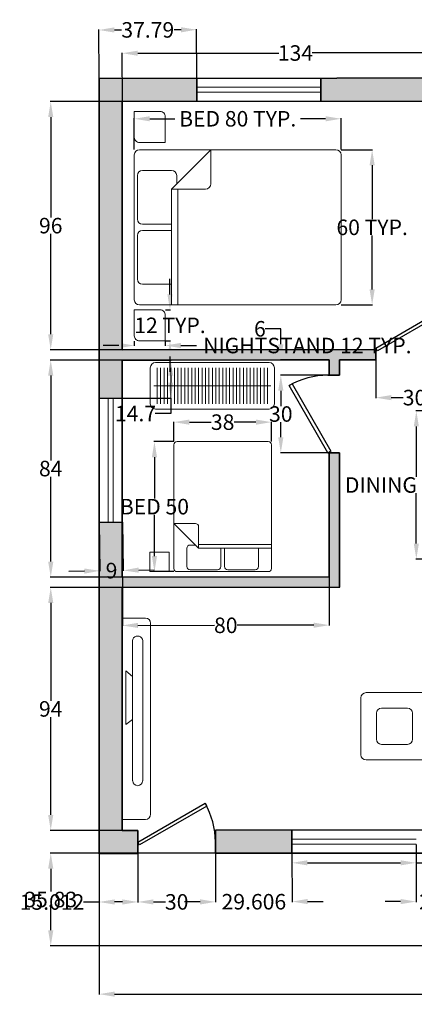
# Model space of a CAD drawing. Units: inches. Extents: x 98 to 487, y -240 to 141.
# Tile 1 of 5: x 98 to 251, y -240 to 141. Entities that reach past the tile are written whole.
import ezdxf

# ---------------------------------------------------------------- set-up
doc = ezdxf.new("R2010")
doc.units = ezdxf.units.IN
doc.header["$MEASUREMENT"] = 0
for name, color, linetype, lineweight in [('A-ANNO-DIMS', 2, 'Continuous', 18), ('A-DOOR', 3, 'Continuous', 25), ('A-EQPM', 9, 'Continuous', 18), ('A-FURN', 8, 'Continuous', 18), ('A-GLAZ', 4, 'Continuous', 18), ('A-WALL', 7, 'Continuous', 35)]:
    doc.layers.add(name, color=color, linetype=linetype, lineweight=lineweight)
doc.layers.add('A-WALL-PATT', color=251, linetype='Continuous', lineweight=13, true_color=0x636466)
doc.styles.get("Standard").update_dxf_attribs({"font": 'arial.ttf'})
doc.dimstyles.get("Standard").update_dxf_attribs({"dimtxt": 6, "dimasz": 6, "dimexe": 0.18, "dimexo": 0.0625, "dimgap": 0.09, "dimtad": 0, "dimtih": 1, "dimtoh": 1, "dimdec": 0, "dimzin": 0, "dimdsep": 46, "dimlunit": 4, "dimtxsty": 'Standard', "dimcen": 0.09, "dimadec": 0, "dimazin": 0, "dimtfac": 1, "dimtdec": 0, "dimtofl": 0, "dimtmove": 0, "dimatfit": 3, "dimfxl": 1, "dimtolj": 1, "dimtzin": 0, "dimarcsym": 0})

# ---------------------------------------------------------------- blocks, each defined once
blk = doc.blocks.new('Bed - Queen')
for p, q in [((2, 0), (57.99999, 0)), ((0, -78.00003), (0, -2)), ((7.99999, -14.4), (7.99999, -3.2)), ((9.99999, -1.2), (26.79998, -1.2)), ((28.79998, -3.2), (28.79998, -14.4)), ((31.19999, -14.4), (31.19999, -3.2)), ((33.19999, -1.2), (49.99999, -1.2)), ((51.99999, -3.2), (51.99999, -14.4)), ((59.99999, -2), (59.99999, -78.00003)), ((0, -14.4), (44.8, -14.4)), ((59.99999, -29.6), (44.8, -14.4)), ((44.8, -14.4), (44.8, -27.6)), ((44.8, -16.8), (0, -16.8)), ((49.99999, -16.4), (46.79936, -16.4)), ((46.8, -29.6), (59.99999, -29.6)), ((57.99999, -80.00003), (2, -80.00003))]:
    blk.add_line(p, q)
for centre, start, end in [((2, -2), 90, 180), ((57.99999, -2), 0, 90), ((9.99999, -3.2), 90, 180), ((26.79998, -3.2), 0, 90), ((33.19999, -3.2), 90, 180), ((49.99999, -3.2), 0, 90), ((49.99999, -14.4), 270, 0), ((46.8, -27.6), 180, 270), ((2, -78.00003), 180, 270), ((57.99999, -78.00003), 270, 0)]:
    blk.add_arc(centre, 2, start, end)
blk = doc.blocks.new('*U8')
for p, q in [((0, 0), (0, -6)), ((40, 0), (40, -6))]:
    blk.add_line(p, q)
blk.add_lwpolyline([(0, 0), (34.64, 20), (35.52, 18.48), (0.87, -1.52)], close=True)
blk.add_arc((0, 0), 40, 0, 30)
blk = doc.blocks.new('GLAZ-48IN')
for p, q in [((48, 2), (0, 2)), ((48, 0), (0, 0))]:
    blk.add_line(p, q)
blk = doc.blocks.new('NIGHTSTAND-12IN-RADIUSED')
blk.add_lwpolyline([(2, 0), (12, 0), (12, 10, 0.414214), (10, 12), (0, 12), (0, 2, 0.414214)], format="xyb", close=True)
blk = doc.blocks.new('WARDROBE-HANGING-RAIL')
for p, q in [((7, 46.67), (7, 1.33)), ((14, 45.33), (0, 45.33)), ((14, 44), (0, 44)), ((14, 42.67), (0, 42.67)), ((14, 41.33), (0, 41.33)), ((14, 40), (0, 40)), ((14, 38.67), (0, 38.67)), ((14, 37.33), (0, 37.33)), ((14, 36), (0, 36)), ((14, 34.67), (0, 34.67)), ((14, 33.33), (0, 33.33)), ((14, 32), (0, 32)), ((14, 30.67), (0, 30.67)), ((14, 29.33), (0, 29.33)), ((14, 28), (0, 28)), ((14, 26.67), (0, 26.67)), ((14, 25.33), (0, 25.33)), ((14, 24), (0, 24)), ((14, 22.67), (0, 22.67)), ((14, 21.33), (0, 21.33)), ((14, 20), (0, 20)), ((14, 18.67), (0, 18.67)), ((14, 17.33), (0, 17.33)), ((14, 16), (0, 16)), ((14, 14.67), (0, 14.67)), ((14, 13.33), (0, 13.33)), ((14, 12), (0, 12)), ((14, 10.67), (0, 10.67)), ((14, 9.33), (0, 9.33)), ((14, 8), (0, 8)), ((14, 6.67), (0, 6.67)), ((14, 5.33), (0, 5.33)), ((14, 4), (0, 4)), ((14, 2.67), (0, 2.67)), ((14, 0), (0, 0))]:
    blk.add_line(p, q)
blk = doc.blocks.new('*D18')
at = {"layer": 'A-ANNO-DIMS', "color": 0, "lineweight": -2, "transparency": 16777216}
for p, q in [((157.66, -22.31), (150, -22.31)), ((150.18, -28.31), (150.18, -44.3)), ((150.18, -66.61), (150.18, -50.61)), ((157.66, -72.61), (150, -72.61))]:
    blk.add_line(p, q, dxfattribs=at)
at = {"layer": 'A-ANNO-DIMS', "color": 0, "transparency": 16777216}
for points in [[(149.18, -28.31), (151.18, -28.31), (150.18, -22.31)], [(149.18, -66.61), (151.18, -66.61), (150.18, -72.61)]]:
    blk.add_solid(points, dxfattribs=at)
at = {"layer": 'Defpoints', "color": 0, "transparency": 16777216}
for p in [(157.72, -22.31), (150.18, -72.61), (157.72, -72.61)]:
    blk.add_point(p, dxfattribs=at)
at = {"layer": 'A-ANNO-DIMS', "color": 0, "transparency": 16777216, "insert": (150.18, -47.46), "char_height": 6, "attachment_point": 5}
blk.add_mtext('\\A1;BED 50', dxfattribs=at)
blk = doc.blocks.new('*D19')
at = {"layer": 'A-ANNO-DIMS', "color": 0, "lineweight": -2, "transparency": 16777216}
for p, q in [((157.72, -22.25), (157.72, -14.58)), ((163.72, -14.76), (172.19, -14.76)), ((189.44, -14.76), (180.97, -14.76)), ((195.44, -22.25), (195.44, -14.58))]:
    blk.add_line(p, q, dxfattribs=at)
at = {"layer": 'A-ANNO-DIMS', "color": 0, "transparency": 16777216}
for points in [[(163.72, -13.76), (163.72, -15.76), (157.72, -14.76)], [(189.44, -13.76), (189.44, -15.76), (195.44, -14.76)]]:
    blk.add_solid(points, dxfattribs=at)
at = {"layer": 'Defpoints', "color": 0, "transparency": 16777216}
for p in [(157.72, -14.76), (157.72, -22.31), (195.44, -22.31)]:
    blk.add_point(p, dxfattribs=at)
at = {"layer": 'A-ANNO-DIMS', "color": 0, "transparency": 16777216, "insert": (176.58, -14.76), "char_height": 6, "attachment_point": 5}
blk.add_mtext('\\A1;38', dxfattribs=at)
blk = doc.blocks.new('*D20')
at = {"layer": 'A-ANNO-DIMS', "color": 0, "lineweight": -2, "transparency": 16777216}
for p, q in [((142.4, 90.68), (142.4, 102.8)), ((148.4, 102.62), (158.05, 102.62)), ((216.4, 102.62), (206.74, 102.62)), ((222.4, 90.68), (222.4, 102.8))]:
    blk.add_line(p, q, dxfattribs=at)
at = {"layer": 'A-ANNO-DIMS', "color": 0, "transparency": 16777216}
for points in [[(148.4, 103.62), (148.4, 101.62), (142.4, 102.62)], [(216.4, 103.62), (216.4, 101.62), (222.4, 102.62)]]:
    blk.add_solid(points, dxfattribs=at)
at = {"layer": 'Defpoints', "color": 0, "transparency": 16777216}
for p in [(142.4, 102.62), (142.4, 90.62), (222.4, 90.62)]:
    blk.add_point(p, dxfattribs=at)
at = {"layer": 'A-ANNO-DIMS', "color": 0, "transparency": 16777216, "insert": (182.4, 102.62), "char_height": 6, "attachment_point": 5}
blk.add_mtext('\\A1;BED 80 TYP.', dxfattribs=at)
blk = doc.blocks.new('*D21')
at = {"layer": 'A-ANNO-DIMS', "color": 0, "lineweight": -2, "transparency": 16777216}
for p, q in [((222.46, 90.62), (234.58, 90.62)), ((234.4, 84.62), (234.4, 63.77)), ((234.4, 36.62), (234.4, 57.46)), ((222.46, 30.62), (234.58, 30.62))]:
    blk.add_line(p, q, dxfattribs=at)
at = {"layer": 'A-ANNO-DIMS', "color": 0, "transparency": 16777216}
for points in [[(233.4, 84.62), (235.4, 84.62), (234.4, 90.62)], [(233.4, 36.62), (235.4, 36.62), (234.4, 30.62)]]:
    blk.add_solid(points, dxfattribs=at)
at = {"layer": 'Defpoints', "color": 0, "transparency": 16777216}
for p in [(222.4, 90.62), (234.4, 90.62), (222.4, 30.62)]:
    blk.add_point(p, dxfattribs=at)
at = {"layer": 'A-ANNO-DIMS', "color": 0, "transparency": 16777216, "insert": (234.4, 60.62), "char_height": 6, "attachment_point": 5}
blk.add_mtext('\\A1;60 TYP.', dxfattribs=at)
blk = doc.blocks.new('*D24')
at = {"layer": 'A-ANNO-DIMS', "color": 0, "lineweight": -2, "transparency": 16777216}
for p, q in [((142.4, 16.63), (142.4, 14.71)), ((154.4, 16.63), (154.4, 14.71)), ((136.4, 14.89), (130.4, 14.89)), ((160.4, 14.89), (166.4, 14.89))]:
    blk.add_line(p, q, dxfattribs=at)
at = {"layer": 'A-ANNO-DIMS', "color": 0, "transparency": 16777216}
for points in [[(136.4, 15.89), (136.4, 13.89), (142.4, 14.89)], [(160.4, 15.89), (160.4, 13.89), (154.4, 14.89)]]:
    blk.add_solid(points, dxfattribs=at)
at = {"layer": 'Defpoints', "color": 0, "transparency": 16777216}
for p in [(142.4, 16.69), (154.4, 16.69), (154.4, 14.89)]:
    blk.add_point(p, dxfattribs=at)
at = {"layer": 'A-ANNO-DIMS', "color": 0, "transparency": 16777216, "insert": (209.35, 14.89), "char_height": 6, "attachment_point": 5}
blk.add_mtext('\\A1;NIGHTSTAND 12 TYP.', dxfattribs=at)
blk = doc.blocks.new('*D25')
at = {"layer": 'A-ANNO-DIMS', "color": 0, "lineweight": -2, "transparency": 16777216}
for p, q in [((156.2, 34.69), (156.2, 40.69)), ((154.46, 28.69), (156.38, 28.69)), ((154.46, 16.69), (156.38, 16.69)), ((156.2, 10.69), (156.2, 4.69))]:
    blk.add_line(p, q, dxfattribs=at)
at = {"layer": 'A-ANNO-DIMS', "color": 0, "transparency": 16777216}
for points in [[(155.2, 34.69), (157.2, 34.69), (156.2, 28.69)], [(155.2, 10.69), (157.2, 10.69), (156.2, 16.69)]]:
    blk.add_solid(points, dxfattribs=at)
at = {"layer": 'Defpoints', "color": 0, "transparency": 16777216}
for p in [(154.4, 28.69), (156.2, 28.69), (154.4, 16.69)]:
    blk.add_point(p, dxfattribs=at)
at = {"layer": 'A-ANNO-DIMS', "color": 0, "transparency": 16777216, "insert": (156.2, 22.69), "char_height": 6, "attachment_point": 5}
blk.add_mtext('\\A1;12 TYP.', dxfattribs=at)
blk = doc.blocks.new('*D28')
at = {"layer": 'A-ANNO-DIMS', "color": 0, "lineweight": -2, "transparency": 16777216}
for p, q in [((203.38, -178.13), (203.38, -185.45)), ((251.38, -178.13), (251.38, -185.45)), ((209.38, -185.27), (245.38, -185.27)), ((251.38, -185.27), (257.38, -185.27))]:
    blk.add_line(p, q, dxfattribs=at)
at = {"layer": 'A-ANNO-DIMS', "color": 0, "transparency": 16777216}
for points in [[(209.38, -184.27), (209.38, -186.27), (203.38, -185.27)], [(245.38, -184.27), (245.38, -186.27), (251.38, -185.27)]]:
    blk.add_solid(points, dxfattribs=at)
at = {"layer": 'Defpoints', "color": 0, "transparency": 16777216}
for p in [(203.38, -178.07), (251.38, -178.07), (251.38, -185.27)]:
    blk.add_point(p, dxfattribs=at)
at = {"layer": 'A-ANNO-DIMS', "color": 0, "transparency": 16777216, "insert": (291.75, -185.27), "char_height": 6, "attachment_point": 5}
blk.add_mtext('\\A1;WINDOW 48 TYP.', dxfattribs=at)
blk = doc.blocks.new('*D38')
at = {"layer": 'A-ANNO-DIMS', "color": 0, "lineweight": -2, "transparency": 16777216}
for p, q in [((260.02, -10.43), (251.31, -10.43)), ((251.49, -16.43), (251.49, -35.89)), ((251.49, -61.73), (251.49, -42.27)), ((260.02, -67.73), (251.31, -67.73))]:
    blk.add_line(p, q, dxfattribs=at)
at = {"layer": 'A-ANNO-DIMS', "color": 0, "transparency": 16777216}
for points in [[(250.49, -16.43), (252.49, -16.43), (251.49, -10.43)], [(250.49, -61.73), (252.49, -61.73), (251.49, -67.73)]]:
    blk.add_solid(points, dxfattribs=at)
at = {"layer": 'Defpoints', "color": 0, "transparency": 16777216}
for p in [(260.09, -10.43), (251.49, -67.73), (260.09, -67.73)]:
    blk.add_point(p, dxfattribs=at)
at = {"layer": 'A-ANNO-DIMS', "color": 0, "transparency": 16777216, "insert": (251.49, -39.08), "char_height": 6, "attachment_point": 5}
blk.add_mtext('\\A1;DINING SET 57', dxfattribs=at)
blk = doc.blocks.new('*D46')
at = {"layer": 'A-ANNO-DIMS', "color": 0, "lineweight": -2, "transparency": 16777216}
for p, q in [((128.77, -181.8), (128.77, -236.26)), ((404.77, -217.44), (404.77, -236.26)), ((134.77, -236.08), (260, -236.08)), ((398.77, -236.08), (273.53, -236.08))]:
    blk.add_line(p, q, dxfattribs=at)
at = {"layer": 'A-ANNO-DIMS', "color": 0, "transparency": 16777216}
for points in [[(134.77, -235.08), (134.77, -237.08), (128.77, -236.08)], [(398.77, -235.08), (398.77, -237.08), (404.77, -236.08)]]:
    blk.add_solid(points, dxfattribs=at)
at = {"layer": 'Defpoints', "color": 0, "transparency": 16777216}
for p in [(128.77, -181.73), (404.77, -217.38), (404.77, -236.08)]:
    blk.add_point(p, dxfattribs=at)
at = {"layer": 'A-ANNO-DIMS', "color": 0, "transparency": 16777216, "insert": (266.77, -236.08), "char_height": 6, "attachment_point": 5}
blk.add_mtext('\\A1;276', dxfattribs=at)
blk = doc.blocks.new('*D48')
at = {"layer": 'A-ANNO-DIMS', "color": 0, "lineweight": -2, "transparency": 16777216}
for p, q in [((166.56, 118.44), (166.5, 137.26)), ((128.77, 118.33), (128.71, 137.15)), ((134.71, 136.99), (137.39, 136.99)), ((160.5, 137.06), (157.82, 137.06))]:
    blk.add_line(p, q, dxfattribs=at)
at = {"layer": 'A-ANNO-DIMS', "color": 0, "transparency": 16777216}
for points in [[(134.71, 137.99), (134.71, 135.99), (128.71, 136.97)], [(160.5, 138.06), (160.5, 136.06), (166.5, 137.08)]]:
    blk.add_solid(points, dxfattribs=at)
at = {"layer": 'Defpoints', "color": 0, "transparency": 16777216}
for p in [(166.5, 137.08), (128.77, 118.27), (166.56, 118.38)]:
    blk.add_point(p, dxfattribs=at)
at = {"layer": 'A-ANNO-DIMS', "color": 0, "transparency": 16777216, "insert": (147.61, 137.02), "char_height": 6, "attachment_point": 5}
blk.add_mtext('\\A1;37.79', dxfattribs=at)
blk = doc.blocks.new('*D50')
at = {"layer": 'A-ANNO-DIMS', "color": 0, "lineweight": -2, "transparency": 16777216}
for p, q in [((137.77, 109.34), (137.74, 128.16)), ((143.74, 127.99), (198.32, 128.06)), ((265.74, 128.15), (211.16, 128.08)), ((271.77, 109.52), (271.74, 128.34))]:
    blk.add_line(p, q, dxfattribs=at)
at = {"layer": 'A-ANNO-DIMS', "color": 0, "transparency": 16777216}
for points in [[(143.74, 128.99), (143.74, 126.99), (137.74, 127.98)], [(265.74, 129.15), (265.74, 127.15), (271.74, 128.16)]]:
    blk.add_solid(points, dxfattribs=at)
at = {"layer": 'Defpoints', "color": 0, "transparency": 16777216}
for p in [(271.74, 128.16), (137.77, 109.28), (271.77, 109.46)]:
    blk.add_point(p, dxfattribs=at)
at = {"layer": 'A-ANNO-DIMS', "color": 0, "transparency": 16777216, "insert": (204.74, 128.07), "char_height": 6, "attachment_point": 5}
blk.add_mtext('\\A1;134', dxfattribs=at)
blk = doc.blocks.new('*D53')
at = {"layer": 'A-ANNO-DIMS', "color": 0, "lineweight": -2, "transparency": 16777216}
for p, q in [((128.77, -53.65), (129.09, -72.46)), ((137.77, -53.49), (138.09, -72.3)), ((123.09, -72.39), (117.09, -72.49)), ((144.09, -72.02), (150.09, -71.92))]:
    blk.add_line(p, q, dxfattribs=at)
at = {"layer": 'A-ANNO-DIMS', "color": 0, "transparency": 16777216}
for points in [[(123.08, -71.39), (123.11, -73.38), (129.09, -72.28)], [(144.07, -71.02), (144.11, -73.02), (138.09, -72.12)]]:
    blk.add_solid(points, dxfattribs=at)
at = {"layer": 'Defpoints', "color": 0, "transparency": 16777216}
for p in [(128.77, -53.58), (137.77, -53.43), (129.09, -72.28)]:
    blk.add_point(p, dxfattribs=at)
at = {"layer": 'A-ANNO-DIMS', "color": 0, "transparency": 16777216, "insert": (133.59, -72.2), "char_height": 6, "attachment_point": 5}
blk.add_mtext('\\A1;9', dxfattribs=at)
blk = doc.blocks.new('*D54')
at = {"layer": 'A-ANNO-DIMS', "color": 0, "lineweight": -2, "transparency": 16777216}
for p, q in [((137.7, 109.28), (109.89, 109.28)), ((110.07, 103.28), (110.07, 64.43)), ((110.07, 19.28), (110.07, 58.13)), ((137.7, 13.28), (109.89, 13.28))]:
    blk.add_line(p, q, dxfattribs=at)
at = {"layer": 'A-ANNO-DIMS', "color": 0, "transparency": 16777216}
for points in [[(109.07, 103.28), (111.07, 103.28), (110.07, 109.28)], [(109.07, 19.28), (111.07, 19.28), (110.07, 13.28)]]:
    blk.add_solid(points, dxfattribs=at)
at = {"layer": 'Defpoints', "color": 0, "transparency": 16777216}
for p in [(137.77, 109.28), (110.07, 13.28), (137.77, 13.28)]:
    blk.add_point(p, dxfattribs=at)
at = {"layer": 'A-ANNO-DIMS', "color": 0, "transparency": 16777216, "insert": (110.07, 61.28), "char_height": 6, "attachment_point": 5}
blk.add_mtext('\\A1;96', dxfattribs=at)
blk = doc.blocks.new('*D55')
at = {"layer": 'A-ANNO-DIMS', "color": 0, "lineweight": -2, "transparency": 16777216}
for p, q in [((137.7, 9.28), (109.89, 9.28)), ((110.07, 3.28), (110.07, -29.57)), ((110.07, -68.72), (110.07, -35.87)), ((137.7, -74.72), (109.89, -74.72))]:
    blk.add_line(p, q, dxfattribs=at)
at = {"layer": 'A-ANNO-DIMS', "color": 0, "transparency": 16777216}
for points in [[(109.07, 3.28), (111.07, 3.28), (110.07, 9.28)], [(109.07, -68.72), (111.07, -68.72), (110.07, -74.72)]]:
    blk.add_solid(points, dxfattribs=at)
at = {"layer": 'Defpoints', "color": 0, "transparency": 16777216}
for p in [(137.77, 9.28), (110.07, -74.72), (137.77, -74.72)]:
    blk.add_point(p, dxfattribs=at)
at = {"layer": 'A-ANNO-DIMS', "color": 0, "transparency": 16777216, "insert": (110.07, -32.72), "char_height": 6, "attachment_point": 5}
blk.add_mtext('\\A1;84', dxfattribs=at)
blk = doc.blocks.new('*D56')
at = {"layer": 'A-ANNO-DIMS', "color": 0, "lineweight": -2, "transparency": 16777216}
for p, q in [((137.77, -74.78), (137.79, -93.6)), ((217.77, -74.68), (217.79, -93.49)), ((143.79, -93.41), (173.41, -93.37)), ((211.79, -93.32), (182.17, -93.36))]:
    blk.add_line(p, q, dxfattribs=at)
at = {"layer": 'A-ANNO-DIMS', "color": 0, "transparency": 16777216}
for points in [[(143.79, -92.41), (143.79, -94.41), (137.79, -93.42)], [(211.79, -92.32), (211.79, -94.32), (217.79, -93.31)]]:
    blk.add_solid(points, dxfattribs=at)
at = {"layer": 'Defpoints', "color": 0, "transparency": 16777216}
for p in [(137.77, -74.72), (217.77, -74.61), (137.79, -93.42)]:
    blk.add_point(p, dxfattribs=at)
at = {"layer": 'A-ANNO-DIMS', "color": 0, "transparency": 16777216, "insert": (177.79, -93.37), "char_height": 6, "attachment_point": 5}
blk.add_mtext('\\A1;80', dxfattribs=at)
blk = doc.blocks.new('*D57')
at = {"layer": 'A-ANNO-DIMS', "color": 0, "lineweight": -2, "transparency": 16777216}
for p, q in [((137.7, -78.72), (109.89, -78.72)), ((110.07, -84.72), (110.07, -122.57)), ((110.07, -166.72), (110.07, -128.87)), ((137.7, -172.72), (109.89, -172.72))]:
    blk.add_line(p, q, dxfattribs=at)
at = {"layer": 'A-ANNO-DIMS', "color": 0, "transparency": 16777216}
for points in [[(109.07, -84.72), (111.07, -84.72), (110.07, -78.72)], [(109.07, -166.72), (111.07, -166.72), (110.07, -172.72)]]:
    blk.add_solid(points, dxfattribs=at)
at = {"layer": 'Defpoints', "color": 0, "transparency": 16777216}
for p in [(137.77, -78.72), (110.07, -172.72), (137.77, -172.72)]:
    blk.add_point(p, dxfattribs=at)
at = {"layer": 'A-ANNO-DIMS', "color": 0, "transparency": 16777216, "insert": (110.07, -125.72), "char_height": 6, "attachment_point": 5}
blk.add_mtext('\\A1;94', dxfattribs=at)
blk = doc.blocks.new('*D58')
at = {"layer": 'A-ANNO-DIMS', "color": 0, "lineweight": -2, "transparency": 16777216}
for p, q in [((278.7, -181.55), (109.89, -181.55)), ((110.07, -187.55), (110.07, -196.31)), ((110.07, -211.38), (110.07, -202.62)), ((278.7, -217.38), (109.89, -217.38))]:
    blk.add_line(p, q, dxfattribs=at)
at = {"layer": 'A-ANNO-DIMS', "color": 0, "transparency": 16777216}
for points in [[(109.07, -187.55), (111.07, -187.55), (110.07, -181.55)], [(109.07, -211.38), (111.07, -211.38), (110.07, -217.38)]]:
    blk.add_solid(points, dxfattribs=at)
at = {"layer": 'Defpoints', "color": 0, "transparency": 16777216}
for p in [(278.77, -181.55), (110.07, -217.38), (278.77, -217.38)]:
    blk.add_point(p, dxfattribs=at)
at = {"layer": 'A-ANNO-DIMS', "color": 0, "transparency": 16777216, "insert": (110.07, -199.46), "char_height": 6, "attachment_point": 5}
blk.add_mtext('\\A1;35.83', dxfattribs=at)
blk = doc.blocks.new('*D59')
at = {"layer": 'A-ANNO-DIMS', "color": 0, "lineweight": -2, "transparency": 16777216}
for p, q in [((128.77, -181.8), (128.79, -200.61)), ((143.78, -181.78), (143.8, -200.59)), ((128.79, -200.43), (122.79, -200.44)), ((137.8, -200.42), (134.79, -200.42))]:
    blk.add_line(p, q, dxfattribs=at)
at = {"layer": 'A-ANNO-DIMS', "color": 0, "transparency": 16777216}
for points in [[(134.79, -199.42), (134.79, -201.42), (128.79, -200.43)], [(137.8, -199.42), (137.8, -201.42), (143.8, -200.41)]]:
    blk.add_solid(points, dxfattribs=at)
at = {"layer": 'Defpoints', "color": 0, "transparency": 16777216}
for p in [(128.77, -181.73), (143.78, -181.71), (128.79, -200.43)]:
    blk.add_point(p, dxfattribs=at)
at = {"layer": 'A-ANNO-DIMS', "color": 0, "transparency": 16777216, "insert": (110.56, -200.44), "char_height": 6, "attachment_point": 5}
blk.add_mtext('\\A1;15.012', dxfattribs=at)
blk = doc.blocks.new('*D60')
at = {"layer": 'A-ANNO-DIMS', "color": 0, "lineweight": -2, "transparency": 16777216}
for p, q in [((143.78, -181.78), (143.8, -200.59)), ((173.78, -181.74), (173.8, -200.55)), ((149.8, -200.4), (154.43, -200.4)), ((167.8, -200.38), (163.18, -200.39))]:
    blk.add_line(p, q, dxfattribs=at)
at = {"layer": 'A-ANNO-DIMS', "color": 0, "transparency": 16777216}
for points in [[(149.8, -199.4), (149.8, -201.4), (143.8, -200.41)], [(167.8, -199.38), (167.8, -201.38), (173.8, -200.37)]]:
    blk.add_solid(points, dxfattribs=at)
at = {"layer": 'Defpoints', "color": 0, "transparency": 16777216}
for p in [(143.78, -181.71), (173.78, -181.67), (143.8, -200.41)]:
    blk.add_point(p, dxfattribs=at)
at = {"layer": 'A-ANNO-DIMS', "color": 0, "transparency": 16777216, "insert": (158.8, -200.39), "char_height": 6, "attachment_point": 5}
blk.add_mtext('\\A1;30', dxfattribs=at)
blk = doc.blocks.new('*D61')
at = {"layer": 'A-ANNO-DIMS', "color": 0, "lineweight": -2, "transparency": 16777216}
for p, q in [((173.78, -181.74), (173.84, -200.55)), ((203.38, -181.63), (203.45, -200.45)), ((167.84, -200.39), (161.84, -200.41)), ((209.45, -200.25), (215.45, -200.23))]:
    blk.add_line(p, q, dxfattribs=at)
at = {"layer": 'A-ANNO-DIMS', "color": 0, "transparency": 16777216}
for points in [[(167.84, -199.39), (167.85, -201.39), (173.84, -200.37)], [(209.44, -199.25), (209.45, -201.25), (203.45, -200.27)]]:
    blk.add_solid(points, dxfattribs=at)
at = {"layer": 'Defpoints', "color": 0, "transparency": 16777216}
for p in [(173.78, -181.67), (203.38, -181.57), (173.84, -200.37)]:
    blk.add_point(p, dxfattribs=at)
at = {"layer": 'A-ANNO-DIMS', "color": 0, "transparency": 16777216, "insert": (188.65, -200.32), "char_height": 6, "attachment_point": 5}
blk.add_mtext('\\A1;29.606', dxfattribs=at)
blk = doc.blocks.new('*D62')
at = {"layer": 'A-ANNO-DIMS', "color": 0, "lineweight": -2, "transparency": 16777216}
for p, q in [((251.38, -181.63), (251.4, -200.45)), ((278.77, -181.61), (278.78, -200.43)), ((245.4, -200.27), (239.4, -200.28)), ((284.78, -200.24), (290.78, -200.24))]:
    blk.add_line(p, q, dxfattribs=at)
at = {"layer": 'A-ANNO-DIMS', "color": 0, "transparency": 16777216}
for points in [[(245.4, -199.27), (245.4, -201.27), (251.4, -200.27)], [(284.78, -199.24), (284.78, -201.24), (278.78, -200.25)]]:
    blk.add_solid(points, dxfattribs=at)
at = {"layer": 'Defpoints', "color": 0, "transparency": 16777216}
for p in [(251.38, -181.57), (278.77, -181.55), (251.4, -200.27)]:
    blk.add_point(p, dxfattribs=at)
at = {"layer": 'A-ANNO-DIMS', "color": 0, "transparency": 16777216, "insert": (265.09, -200.26), "char_height": 6, "attachment_point": 5}
blk.add_mtext('\\A1;27.383', dxfattribs=at)
blk = doc.blocks.new('*D71')
at = {"layer": 'A-ANNO-DIMS', "color": 0, "lineweight": -2, "transparency": 16777216}
for p, q in [((235.77, 13.35), (235.79, -5.47)), ((265.77, 13.39), (265.79, -5.43)), ((241.79, -5.28), (246.42, -5.28)), ((259.79, -5.26), (255.17, -5.26))]:
    blk.add_line(p, q, dxfattribs=at)
at = {"layer": 'A-ANNO-DIMS', "color": 0, "transparency": 16777216}
for points in [[(241.79, -4.28), (241.79, -6.28), (235.79, -5.29)], [(259.79, -4.26), (259.79, -6.26), (265.79, -5.25)]]:
    blk.add_solid(points, dxfattribs=at)
at = {"layer": 'Defpoints', "color": 0, "transparency": 16777216}
for p in [(235.77, 13.41), (265.77, 13.45), (235.79, -5.29)]:
    blk.add_point(p, dxfattribs=at)
at = {"layer": 'A-ANNO-DIMS', "color": 0, "transparency": 16777216, "insert": (250.79, -5.27), "char_height": 6, "attachment_point": 5}
blk.add_mtext('\\A1;30', dxfattribs=at)
blk = doc.blocks.new('*D78')
at = {"layer": 'A-ANNO-DIMS', "color": 0, "lineweight": -2, "transparency": 16777216}
for p, q in [((137.83, 9.28), (156.65, 9.28)), ((156.47, 3.28), (156.47, 0.58)), ((137.83, -5.42), (156.65, -5.42)), ((156.47, -5.42), (156.47, -11.42)), ((156.47, -11.42), (150.47, -11.42))]:
    blk.add_line(p, q, dxfattribs=at)
at = {"layer": 'A-ANNO-DIMS', "color": 0, "transparency": 16777216}
for points in [[(155.47, 3.28), (157.47, 3.28), (156.47, 9.28)], [(155.47, 0.58), (157.47, 0.58), (156.47, -5.42)]]:
    blk.add_solid(points, dxfattribs=at)
at = {"layer": 'Defpoints', "color": 0, "transparency": 16777216}
for p in [(137.77, 9.28), (137.77, -5.42), (156.47, -5.42)]:
    blk.add_point(p, dxfattribs=at)
at = {"layer": 'A-ANNO-DIMS', "color": 0, "transparency": 16777216, "insert": (142.87, -11.42), "char_height": 6, "attachment_point": 5}
blk.add_mtext('\\A1;14.7', dxfattribs=at)
blk = doc.blocks.new('*D82')
at = {"layer": 'A-ANNO-DIMS', "color": 0, "lineweight": -2, "transparency": 16777216}
for p, q in [((199.05, 21.36), (193.05, 21.36)), ((199.06, 15.36), (199.05, 21.36)), ((217.7, 9.39), (198.89, 9.36)), ((217.71, 3.39), (198.89, 3.36)), ((199.08, -2.64), (199.09, -8.64))]:
    blk.add_line(p, q, dxfattribs=at)
at = {"layer": 'A-ANNO-DIMS', "color": 0, "transparency": 16777216}
for points in [[(200.06, 15.36), (198.06, 15.36), (199.07, 9.36)], [(200.08, -2.64), (198.08, -2.64), (199.07, 3.36)]]:
    blk.add_solid(points, dxfattribs=at)
at = {"layer": 'Defpoints', "color": 0, "transparency": 16777216}
for p in [(199.07, 9.36), (217.77, 9.39), (217.77, 3.39)]:
    blk.add_point(p, dxfattribs=at)
at = {"layer": 'A-ANNO-DIMS', "color": 0, "transparency": 16777216, "insert": (190.98, 21.36), "char_height": 6, "attachment_point": 5}
blk.add_mtext('\\A1;6', dxfattribs=at)
blk = doc.blocks.new('*D83')
at = {"layer": 'A-ANNO-DIMS', "color": 0, "lineweight": -2, "transparency": 16777216}
for p, q in [((217.71, 3.39), (198.89, 3.39)), ((199.07, -2.61), (199.07, -8.45)), ((199.07, -20.61), (199.07, -14.76)), ((217.7, -26.61), (198.89, -26.61))]:
    blk.add_line(p, q, dxfattribs=at)
at = {"layer": 'A-ANNO-DIMS', "color": 0, "transparency": 16777216}
for points in [[(198.07, -2.61), (200.07, -2.61), (199.07, 3.39)], [(198.07, -20.61), (200.07, -20.61), (199.07, -26.61)]]:
    blk.add_solid(points, dxfattribs=at)
at = {"layer": 'Defpoints', "color": 0, "transparency": 16777216}
for p in [(199.07, 3.39), (217.77, 3.39), (217.77, -26.61)]:
    blk.add_point(p, dxfattribs=at)
at = {"layer": 'A-ANNO-DIMS', "color": 0, "transparency": 16777216, "insert": (199.07, -11.61), "char_height": 6, "attachment_point": 5}
blk.add_mtext('\\A1;30', dxfattribs=at)

msp = doc.modelspace()

# ---------------------------------------------------------------- hatches: boundary and pattern name
at = {"layer": 'A-WALL-PATT'}
h = msp.add_hatch(color=256, dxfattribs=at)
h.dxf.hatch_style = 1
h.paths.add_polyline_path([(137.7655, 9.279), (217.7655, 9.3857), (217.7735, 3.391), (221.7455, 3.391), (221.7655, 3.391), (221.7655, 9.391), (221.7717, 9.391), (235.7717, 9.4097), (235.7663, 13.4097), (137.7655, 13.279), (137.7655, 109.2791), (166.5584, 109.3175), (166.5584, 118.3175), (128.7655, 118.2671), (128.7655, -5.5765), (137.7655, -5.4202)])
h = msp.add_hatch(color=256, dxfattribs=at)
h.dxf.hatch_style = 1
h.paths.add_polyline_path([(316.6174, 118.5177), (214.5584, 118.3815), (214.5584, 109.3815), (271.7663, 109.4578), (271.7663, 13.4577), (265.7717, 13.4497), (265.7717, 9.4497), (271.7663, 9.4577), (281.7716, 9.4711), (281.7663, 13.4711), (275.7663, 13.4631), (275.7663, 109.4632), (316.6174, 109.5177)])
h = msp.add_hatch(color=256, dxfattribs=at)
h.dxf.hatch_style = 1
h.paths.add_polyline_path([(137.7655, -53.4275), (128.7655, -53.5838), (128.7655, -181.7329), (143.7775, -181.7129), (143.7655, -172.7129), (137.7655, -172.7209), (137.7655, -78.7211), (221.7655, -78.609), (221.7655, -26.609), (217.7655, -26.6143), (217.7655, -74.6144), (137.7655, -74.7211)])
h = msp.add_hatch(color=256, dxfattribs=at)
h.dxf.hatch_style = 1
h.paths.add_polyline_path([(203.3829, -172.6334), (173.7655, -172.6729), (173.7707, -176.5728, -0.00533515), (173.7775, -177.2129), (173.7775, -181.6729), (203.3829, -181.6334)])

# ---------------------------------------------------------------- linework, layer by layer
at = {"layer": 'A-EQPM'}
msp.add_line((139.1809, -131.7814), (141.6971, -129.8714), dxfattribs=at)
for points in [[(141.7697, -153.5249), (141.6971, -153.5249), (141.6971, -99.5349)], [(145.6519, -99.5349), (145.6519, -153.5249), (145.5793, -153.5249)], [(139.1809, -131.7814), (139.1809, -111.0208), (141.6971, -113.1937)], [(141.6971, -111.0208), (141.6971, -131.7814)]]:
    msp.add_lwpolyline(points, dxfattribs=at)
for centre, radius, start, end in [((143.6745, -99.5349), 2.0188, 348.379925, 191.620075), ((143.6745, -153.5249), 1.9048, 180, 0)]:
    msp.add_arc(centre, radius, start, end, dxfattribs=at)
at = {"layer": 'A-FURN'}
for points in [[(194.5901, -9.6959), (150.5901, -9.6959, -0.41421356), (148.5901, -7.6959), (148.5901, 6.3041, -0.41421356), (150.5901, 8.3041), (194.5901, 8.3041, -0.41421356), (196.5901, 6.3041), (196.5901, -7.6959, -0.41421356)], [(137.7655, -90.5454), (146.7029, -90.5454, -0.41421356), (148.7029, -92.5454), (148.7029, -166.4777, -0.41421356), (146.7029, -168.4777), (137.7655, -168.4777)], [(254.0396, -119.4274), (232.0396, -119.4274, 0.41421356), (230.0396, -121.4274), (230.0396, -143.4274, 0.41421356), (232.0396, -145.4274), (254.0396, -145.4274, 0.41421356), (256.0396, -143.4274), (256.0396, -121.4274, 0.41421356)], [(248.0396, -125.4274), (238.0396, -125.4274, 0.41421356), (236.0396, -127.4274), (236.0396, -137.4274, 0.41421356), (238.0396, -139.4274), (248.0396, -139.4274, 0.41421356), (250.0396, -137.4274), (250.0396, -127.4274, 0.41421356)]]:
    msp.add_lwpolyline(points, format="xyb", close=True, dxfattribs=at)
msp.add_lwpolyline([(155.941, -72.6074), (155.941, -65.0627), (148.3963, -65.0627), (148.3963, -72.6074)], close=True, dxfattribs=at)
at = {"layer": 'A-GLAZ'}
for p, q in [((132.2655, -5.4984), (132.2662, -53.5056)), ((134.2655, -5.4984), (134.2662, -53.5056))]:
    msp.add_line(p, q, dxfattribs=at)
at = {"layer": 'A-WALL'}
for p, q in [((166.5584, 109.3815), (166.5584, 118.3815)), ((214.5584, 118.3815), (214.5584, 109.3815)), ((137.7655, 109.2791), (271.7663, 109.4578)), ((137.7655, 13.279), (137.7655, 109.2791)), ((137.7655, 13.279), (235.7663, 13.4097)), ((235.7663, 13.4097), (235.7717, 9.4097)), ((137.7655, 9.279), (217.7655, 9.3857)), ((137.7655, -74.7211), (137.7655, 9.279)), ((217.7655, 9.3857), (217.7735, 3.3857)), ((221.7655, 9.391), (221.7717, 9.391)), ((221.7655, 3.391), (221.7655, 9.391)), ((235.7717, 9.4097), (221.7717, 9.391)), ((217.7735, 3.3857), (221.7797, 3.391)), ((128.7655, -5.5765), (137.7655, -5.4202)), ((217.7655, -26.6143), (221.8197, -26.6089)), ((217.7655, -74.6144), (217.7655, -26.6143)), ((221.7655, -78.609), (221.7655, -26.609)), ((137.7655, -53.4275), (128.7669, -53.5837)), ((137.7655, -74.7211), (217.7655, -74.6144)), ((221.7655, -74.609), (221.8837, -74.6089)), ((137.7655, -78.7211), (221.8891, -78.6089)), ((137.7655, -172.7209), (137.7655, -78.7211)), ((143.7655, -172.7129), (137.7655, -172.7209)), ((143.7655, -172.7129), (143.7775, -181.7129)), ((271.7663, -172.5422), (173.7655, -172.6729)), ((173.7655, -172.6729), (173.7775, -181.6729)), ((203.3829, -181.5694), (203.3829, -172.5694)), ((217.7655, -172.7209), (217.7655, -172.6142)), ((221.7655, -172.7209), (221.7655, -172.6089))]:
    msp.add_line(p, q, dxfattribs=at)
for points in [[(143.7775, -181.7129), (128.7655, -181.7329), (128.7655, 118.2671), (404.7663, 118.6353), (404.7663, -181.3647)], [(266.7305, -181.5489), (173.7775, -181.6729)]]:
    msp.add_lwpolyline(points, dxfattribs=at)

# ---------------------------------------------------------------- block references
at = {"layer": 'A-DOOR', "xscale": 0.75, "yscale": 0.75, "zscale": 0.75}
for p in [(235.7717, 13.9097), (143.7775, -177.2129)]:
    msp.add_blockref('*U8', p, dxfattribs=at)
at = {"layer": 'A-DOOR', "xscale": 0.75, "yscale": 0.75, "zscale": 0.75, "rotation": 90}
msp.add_blockref('*U8', (217.2655, -26.609), dxfattribs=at)
at = {"layer": 'A-FURN'}
for p in [(142.396, 93.447), (142.396, 16.6926)]:
    msp.add_blockref('NIGHTSTAND-12IN-RADIUSED', p, dxfattribs=at)
for name, p, rotation in [('Bed - Queen', (142.3965, 30.6162), 90), ('WARDROBE-HANGING-RAIL', (148.5905, 6.3036), 270.0000000000001)]:
    msp.add_blockref(name, p, dxfattribs=dict(at, rotation=rotation))
at = {"layer": 'A-FURN', "xscale": 0.6287254313149208, "yscale": 0.6287254313149208, "zscale": 0.6287254313149208, "rotation": 180}
msp.add_blockref('Bed - Queen', (195.4442, -72.6074), dxfattribs=at)
at = {"layer": 'A-GLAZ'}
for p in [(166.558, 112.882), (203.3825, -178.0689)]:
    msp.add_blockref('GLAZ-48IN', p, dxfattribs=at)

# ---------------------------------------------------------------- dimensions: what is measured, and where the dimension line sits
at = {"layer": 'A-ANNO-DIMS'}
for base, p1, p2, angle, override, picture, middle in [((166.5018, 137.0814), (128.7655, 118.2671), (166.5584, 118.3815), 0.173512, {"dimdec": 2, "dimlfac": 1, "dimrnd": 0, "dimzin": 0, "dimdsep": 46, "dimlunit": 2}, '*D48', (147.6053, 137.0242)), ((271.7414, 128.1578), (137.7655, 109.2791), (271.7663, 109.4578), 0.07644, {"dimdec": 0, "dimlfac": 1, "dimrnd": 0, "dimzin": 0, "dimdsep": 46, "dimlunit": 2}, '*D50', (204.7409, 128.0684)), ((110.0655, 13.279), (137.7655, 109.2791), (137.7655, 13.279), 90, {"dimdec": 0, "dimlfac": 1, "dimrnd": 0, "dimzin": 0, "dimdsep": 46, "dimlunit": 2}, '*D54', (110.0655, 61.279)), ((199.0655, 9.3607), (217.7735, 3.3857), (217.7655, 9.3857), 90.07644, {"dimdec": 0, "dimlfac": 1, "dimrnd": 0, "dimzin": 0, "dimdsep": 46, "dimlunit": 2}, '*D82', (190.9786, 21.3607)), ((235.7913, -5.2903), (265.7663, 13.4497), (235.7663, 13.4097), 180.07644, {"dimdec": 0, "dimlfac": 1, "dimrnd": 0, "dimzin": 0, "dimdsep": 46, "dimlunit": 2}, '*D71', (250.7913, -5.2703)), ((110.0655, -74.7211), (137.7655, 9.279), (137.7655, -74.7211), 90, {"dimdec": 0, "dimlfac": 1, "dimrnd": 0, "dimzin": 0, "dimdsep": 46, "dimlunit": 2}, '*D55', (110.0655, -32.7211)), ((156.4655, -5.4202), (137.7655, 9.279), (137.7655, -5.4202), 270, {"dimdec": 1, "dimlfac": 1, "dimrnd": 0, "dimzin": 0, "dimdsep": 46, "dimlunit": 2}, '*D78', (142.8653, -11.4202)), ((199.0735, 3.3907), (217.7655, -26.6143), (217.7735, 3.3857), 89.984712, {"dimdec": 0, "dimlfac": 1, "dimrnd": 0, "dimzin": 0, "dimdsep": 46, "dimlunit": 2}, '*D83', (199.0695, -11.6093)), ((157.7207, -14.7646), (195.4442, -22.3093), (157.7207, -22.3093), 180, {"dimdec": 0, "dimlfac": 1, "dimrnd": 0, "dimzin": 0, "dimdsep": 46, "dimlunit": 2}, '*D19', (176.5825, -14.7646)), ((129.0915, -72.2809), (137.7655, -53.4275), (128.7669, -53.5837), 180.994797, {"dimdec": 0, "dimlfac": 1, "dimrnd": 0, "dimzin": 0, "dimdsep": 46, "dimlunit": 2}, '*D53', (133.5908, -72.2028)), ((137.7904, -93.4211), (217.7655, -74.6144), (137.7655, -74.7211), 180.07644, {"dimdec": 0, "dimlfac": 1, "dimrnd": 0, "dimzin": 0, "dimdsep": 46, "dimlunit": 2}, '*D56', (177.7904, -93.3677)), ((110.0655, -172.7209), (137.7655, -78.7211), (137.7655, -172.7209), 90, {"dimdec": 0, "dimlfac": 1, "dimrnd": 0, "dimzin": 0, "dimdsep": 46, "dimlunit": 2}, '*D57', (110.0655, -125.721)), ((128.7904, -200.4329), (143.7775, -181.7129), (128.7655, -181.7329), 180.07644, {"dimdec": 3, "dimlfac": 1, "dimrnd": 0, "dimzin": 0, "dimdsep": 46, "dimlunit": 2}, '*D59', (110.5592, -200.4409)), ((110.0655, -217.3767), (278.7663, -181.5489), (278.7663, -217.3767), 90, {"dimdec": 2, "dimlfac": 1, "dimrnd": 0, "dimzin": 0, "dimdsep": 46, "dimlunit": 2}, '*D58', (110.0655, -199.4628)), ((143.8024, -200.4129), (173.7775, -181.6729), (143.7775, -181.7129), 180.07644, {"dimdec": 0, "dimlfac": 1, "dimrnd": 0, "dimzin": 0, "dimdsep": 46, "dimlunit": 2}, '*D60', (158.8024, -200.3929)), ((173.8429, -200.3728), (203.3829, -181.5694), (173.7775, -181.6729), 180.200373, {"dimdec": 3, "dimlfac": 1, "dimrnd": 0, "dimzin": 0, "dimdsep": 46, "dimlunit": 2}, '*D61', (188.6456, -200.321)), ((251.3968, -200.2694), (278.7663, -181.5489), (251.3829, -181.5694), 180.042842, {"dimdec": 3, "dimlfac": 1, "dimrnd": 0, "dimzin": 0, "dimdsep": 46, "dimlunit": 2}, '*D62', (265.0886, -200.2591))]:
    dim = msp.add_linear_dim(base=base, p1=p1, p2=p2, angle=angle, dimstyle='Standard', override=override, dxfattribs=at)
    dim.commit()
    dim.dimension.update_dxf_attribs({"geometry": picture, "text_midpoint": middle})
for base, p1, p2, angle, text, picture, middle in [((142.3965, 102.6162), (222.3965, 90.6162), (142.3965, 90.6162), 180, 'BED <> TYP.', '*D20', (182.3965, 102.6162)), ((234.3965, 90.6162), (222.3965, 30.6162), (222.3965, 90.6162), 90, '<> TYP.', '*D21', (234.3965, 60.6162)), ((156.1965, 28.6923), (154.3965, 16.6923), (154.3965, 28.6923), 90, '<> TYP.', '*D25', (156.1965, 22.6923)), ((251.4905, -67.7331), (260.0867, -10.4252), (260.0867, -67.7331), 270, 'DINING SET <>', '*D38', (251.4905, -39.0791)), ((150.176, -72.6074), (157.7207, -22.3093), (157.7207, -72.6074), 270, 'BED <>', '*D18', (150.176, -47.4584))]:
    dim = msp.add_linear_dim(base=base, p1=p1, p2=p2, angle=angle, text=text, dimstyle='Standard', override={"dimdec": 0, "dimlfac": 1, "dimrnd": 0, "dimzin": 0, "dimdsep": 46, "dimlunit": 2}, dxfattribs=at)
    dim.commit()
    dim.dimension.update_dxf_attribs({"geometry": picture, "text_midpoint": middle})
for base, p1, p2, text, picture, middle in [((154.3965, 14.8923), (142.3965, 16.6923), (154.3965, 16.6923), 'NIGHTSTAND <> TYP.', '*D24', (209.3501, 14.8923)), ((251.3829, -185.2694), (203.3829, -178.0694), (251.3829, -178.0694), 'WINDOW <> TYP.', '*D28', (291.7519, -185.2694))]:
    dim = msp.add_linear_dim(base=base, p1=p1, p2=p2, text=text, dimstyle='Standard', override={"dimdec": 0, "dimlfac": 1, "dimrnd": 0, "dimzin": 0, "dimdsep": 46, "dimlunit": 2}, dxfattribs=at)
    dim.commit()
    dim.dimension.update_dxf_attribs({"geometry": picture, "text_midpoint": middle})
dim = msp.add_linear_dim(base=(404.7663, -236.0767), p1=(128.7655, -181.7329), p2=(404.7663, -217.3767), dimstyle='Standard', override={"dimdec": 0, "dimlfac": 1, "dimrnd": 0, "dimzin": 0, "dimdsep": 46, "dimlunit": 2}, dxfattribs=at)
dim.commit()
dim.dimension.update_dxf_attribs({"geometry": '*D46', "text_midpoint": (266.7659, -236.0767)})

doc.saveas('drawing.dxf')
